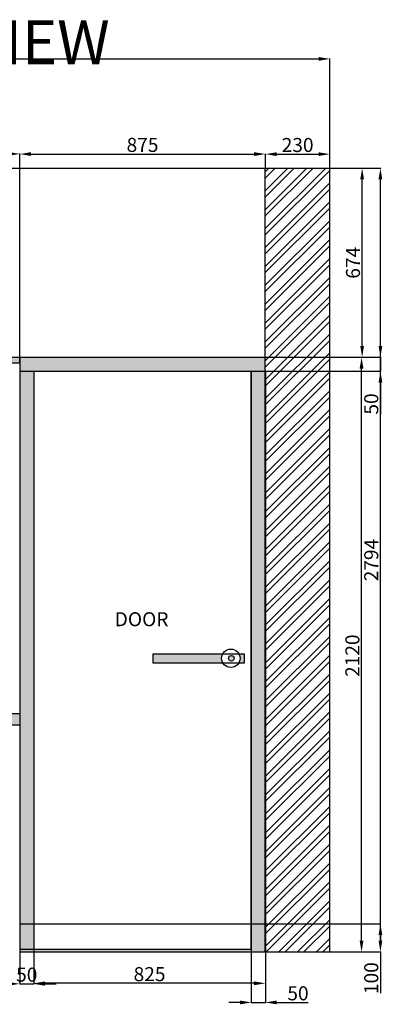
# Model space of a CAD drawing. Units: millimetres. Extents: x 144895 to 155057, y -2833 to 1092.
# Tile 2 of 4: x 147257 to 148549, y -2807 to 703. Entities that reach past the tile are written whole.
import ezdxf

# ---------------------------------------------------------------- set-up
doc = ezdxf.new("R2010")
doc.units = ezdxf.units.MM
for name, color, linetype, lineweight in [('A-ANNO-DIMS', 2, 'Continuous', 18), ('A-ANNO-TEXT', 7, 'Continuous', 18), ('A-DOOR', 4, 'Continuous', 25), ('A-ELEV', 7, 'Continuous', 25), ('A-ELEV-PATT', 252, 'Continuous', 13), ('A-WALL-PATT', 8, 'Continuous', 13)]:
    doc.layers.add(name, color=color, linetype=linetype, lineweight=lineweight)
doc.styles.get("Standard").update_dxf_attribs({"font": 'arial.ttf'})
doc.dimstyles.new('ISO-25', dxfattribs={"dimtxt": 50, "dimasz": 40, "dimexe": 1.25, "dimexo": 0.625, "dimtad": 1, "dimtxsty": 'Standard', "dimcen": 2.5, "dimadec": 0, "dimazin": 0, "dimtfac": 1, "dimtmove": 0, "dimatfit": 3, "dimfxl": 1, "dimarcsym": 0})

# ---------------------------------------------------------------- blocks, each defined once
blk = doc.blocks.new('*D13')
at = {"layer": 'A-ANNO-DIMS', "color": 0, "lineweight": -2, "transparency": 16777216}
for p, q in [((147257.5, -2621.3), (147257.5, -2735.6)), ((147307.5, -2621.3), (147307.5, -2735.6)), ((147217.5, -2734.4), (147177.5, -2734.4)), ((147257.5, -2734.4), (147307.5, -2734.4)), ((147347.5, -2734.4), (147387.5, -2734.4))]:
    blk.add_line(p, q, dxfattribs=at)
at = {"layer": 'A-ANNO-DIMS', "color": 0, "transparency": 16777216}
for points in [[(147217.5, -2727.7), (147217.5, -2741.1), (147257.5, -2734.4)], [(147347.5, -2727.7), (147347.5, -2741.1), (147307.5, -2734.4)]]:
    blk.add_solid(points, dxfattribs=at)
at = {"layer": 'Defpoints', "color": 0, "transparency": 16777216}
for p in [(147257.5, -2620.7), (147307.5, -2620.7), (147307.5, -2734.4)]:
    blk.add_point(p, dxfattribs=at)
at = {"layer": 'A-ANNO-DIMS', "color": 0, "transparency": 16777216, "insert": (147282.5, -2708.2), "char_height": 50, "attachment_point": 5}
blk.add_mtext('50', dxfattribs=at)
blk = doc.blocks.new('*D14')
at = {"layer": 'A-ANNO-DIMS', "color": 0, "lineweight": -2, "transparency": 16777216}
for p, q in [((147307.5, -2621.3), (147307.5, -2733.7)), ((148132.5, -2621.3), (148132.5, -2733.7)), ((148092.5, -2732.5), (147347.5, -2732.5))]:
    blk.add_line(p, q, dxfattribs=at)
at = {"layer": 'A-ANNO-DIMS', "color": 0, "transparency": 16777216}
for points in [[(147347.5, -2725.8), (147347.5, -2739.2), (147307.5, -2732.5)], [(148092.5, -2725.8), (148092.5, -2739.2), (148132.5, -2732.5)]]:
    blk.add_solid(points, dxfattribs=at)
at = {"layer": 'Defpoints', "color": 0, "transparency": 16777216}
for p in [(147307.5, -2620.7), (148132.5, -2620.7), (147307.5, -2732.5)]:
    blk.add_point(p, dxfattribs=at)
at = {"layer": 'A-ANNO-DIMS', "color": 0, "transparency": 16777216, "insert": (147720, -2706.3), "char_height": 50, "attachment_point": 5}
blk.add_mtext('825', dxfattribs=at)
blk = doc.blocks.new('*D22')
at = {"layer": 'A-ANNO-DIMS', "color": 0, "lineweight": -2, "ltscale": 20, "transparency": 16777216}
for p, q in [((146794.5, 173.9), (146794.5, 225.6)), ((147217.5, 224.4), (146834.5, 224.4)), ((147257.5, 173.9), (147257.5, 225.6))]:
    blk.add_line(p, q, dxfattribs=at)
at = {"layer": 'A-ANNO-DIMS', "color": 0, "ltscale": 20, "transparency": 16777216}
for points in [[(146834.5, 231), (146834.5, 217.7), (146794.5, 224.4)], [(147217.5, 231), (147217.5, 217.7), (147257.5, 224.4)]]:
    blk.add_solid(points, dxfattribs=at)
at = {"layer": 'Defpoints', "color": 0, "ltscale": 20, "transparency": 16777216}
for p in [(146794.5, 224.4), (146794.5, 173.3), (147257.5, 173.3)]:
    blk.add_point(p, dxfattribs=at)
at = {"layer": 'A-ANNO-DIMS', "color": 0, "ltscale": 20, "transparency": 16777216, "insert": (147026, 250.6), "char_height": 50, "attachment_point": 5}
blk.add_mtext('463', dxfattribs=at)
blk = doc.blocks.new('*D24')
at = {"layer": 'A-ANNO-DIMS', "color": 0, "lineweight": -2, "ltscale": 20, "transparency": 16777216}
for p, q in [((148131.9, -500.7), (148476.5, -500.7)), ((148475.2, -2580.7), (148475.2, -540.7)), ((148133.1, -2620.7), (148476.5, -2620.7))]:
    blk.add_line(p, q, dxfattribs=at)
at = {"layer": 'A-ANNO-DIMS', "color": 0, "ltscale": 20, "transparency": 16777216}
for points in [[(148468.5, -540.7), (148481.9, -540.7), (148475.2, -500.7)], [(148468.5, -2580.7), (148481.9, -2580.7), (148475.2, -2620.7)]]:
    blk.add_solid(points, dxfattribs=at)
at = {"layer": 'Defpoints', "color": 0, "ltscale": 20, "transparency": 16777216}
for p in [(148131.3, -500.7), (148475.2, -500.7), (148132.5, -2620.7)]:
    blk.add_point(p, dxfattribs=at)
at = {"layer": 'A-ANNO-DIMS', "color": 0, "ltscale": 20, "transparency": 16777216, "insert": (148449.1, -1564.5), "char_height": 50, "attachment_point": 5, "rotation": 90}
blk.add_mtext('2120', dxfattribs=at)
blk = doc.blocks.new('*D25')
at = {"layer": 'A-ANNO-DIMS', "color": 0, "lineweight": -2, "ltscale": 20, "transparency": 16777216}
for p, q in [((148131.9, 173.3), (148478.6, 173.3)), ((148477.3, -460.7), (148477.3, 133.3)), ((148131.9, -500.7), (148478.6, -500.7))]:
    blk.add_line(p, q, dxfattribs=at)
at = {"layer": 'A-ANNO-DIMS', "color": 0, "ltscale": 20, "transparency": 16777216}
for points in [[(148470.7, 133.3), (148484, 133.3), (148477.3, 173.3)], [(148470.7, -460.7), (148484, -460.7), (148477.3, -500.7)]]:
    blk.add_solid(points, dxfattribs=at)
at = {"layer": 'Defpoints', "color": 0, "ltscale": 20, "transparency": 16777216}
for p in [(148131.3, 173.3), (148477.3, 173.3), (148131.3, -500.7)]:
    blk.add_point(p, dxfattribs=at)
at = {"layer": 'A-ANNO-DIMS', "color": 0, "ltscale": 20, "transparency": 16777216, "insert": (148451.2, -163.7), "char_height": 50, "attachment_point": 5, "rotation": 90}
blk.add_mtext('674', dxfattribs=at)
blk = doc.blocks.new('*D26')
at = {"layer": 'A-ANNO-DIMS', "color": 0, "lineweight": -2, "ltscale": 20, "transparency": 16777216}
for p, q in [((147257.5, 173.9), (147257.5, 225.1)), ((147297.5, 223.8), (148092.5, 223.8)), ((148132.5, 173.9), (148132.5, 225.1))]:
    blk.add_line(p, q, dxfattribs=at)
at = {"layer": 'A-ANNO-DIMS', "color": 0, "ltscale": 20, "transparency": 16777216}
for points in [[(147297.5, 230.5), (147297.5, 217.1), (147257.5, 223.8)], [(148092.5, 230.5), (148092.5, 217.1), (148132.5, 223.8)]]:
    blk.add_solid(points, dxfattribs=at)
at = {"layer": 'Defpoints', "color": 0, "ltscale": 20, "transparency": 16777216}
for p in [(148132.5, 223.8), (147257.5, 173.3), (148132.5, 173.3)]:
    blk.add_point(p, dxfattribs=at)
at = {"layer": 'A-ANNO-DIMS', "color": 0, "ltscale": 20, "transparency": 16777216, "insert": (147695, 250), "char_height": 50, "attachment_point": 5}
blk.add_mtext('875', dxfattribs=at)
blk = doc.blocks.new('*D27')
at = {"layer": 'A-ANNO-DIMS', "color": 0, "lineweight": -2, "ltscale": 20, "transparency": 16777216}
for p, q in [((148132.5, 173.9), (148132.5, 224.8)), ((148172.5, 223.6), (148322.5, 223.6)), ((148362.5, 173.9), (148362.5, 224.8))]:
    blk.add_line(p, q, dxfattribs=at)
at = {"layer": 'A-ANNO-DIMS', "color": 0, "ltscale": 20, "transparency": 16777216}
for points in [[(148172.5, 230.2), (148172.5, 216.9), (148132.5, 223.6)], [(148322.5, 230.2), (148322.5, 216.9), (148362.5, 223.6)]]:
    blk.add_solid(points, dxfattribs=at)
at = {"layer": 'Defpoints', "color": 0, "ltscale": 20, "transparency": 16777216}
for p in [(148362.5, 223.6), (148132.5, 173.3), (148362.5, 173.3)]:
    blk.add_point(p, dxfattribs=at)
at = {"layer": 'A-ANNO-DIMS', "color": 0, "ltscale": 20, "transparency": 16777216, "insert": (148247.5, 249.7), "char_height": 50, "attachment_point": 5}
blk.add_mtext('230', dxfattribs=at)
blk = doc.blocks.new('DOOR-HANDLE')
at = {"ltscale": 20}
h = blk.add_hatch(color=256, dxfattribs=at)
h.dxf.hatch_style = 1
h.paths.add_polyline_path([(147980.9, -1557.7), (147732.7, -1557.7), (147732.7, -1591.4), (147982, -1591.4, -0.143725), (147976.8, -1573.6, -0.127114)])
h.paths.add_polyline_path([(148056.8, -1557.7), (148038.3, -1557.7, -0.127123), (148042.5, -1573.6, -0.143716), (148037.2, -1591.4), (148056.8, -1591.4)])
h.paths.add_polyline_path([(148001.6, -1573.7, 1), (148021.1, -1573.7, 1)])
blk.add_lwpolyline([(147732.7, -1557.7), (148056.8, -1557.7), (148056.8, -1591.4), (147732.7, -1591.4)], close=True, dxfattribs=at)
for centre, radius in [((148009.6, -1573.6), 32.8), ((148011.4, -1573.7), 9.79)]:
    blk.add_circle(centre, radius, dxfattribs=at)
blk = doc.blocks.new('*D46')
at = {"layer": 'A-ANNO-DIMS', "color": 0, "lineweight": -2, "ltscale": 20, "transparency": 16777216}
for p, q in [((145137.5, 173.9), (145137.5, 564.4)), ((145177.5, 563.2), (148322.5, 563.2)), ((148362.5, 173.9), (148362.5, 564.4))]:
    blk.add_line(p, q, dxfattribs=at)
at = {"layer": 'A-ANNO-DIMS', "color": 0, "ltscale": 20, "transparency": 16777216}
for points in [[(145177.5, 569.8), (145177.5, 556.5), (145137.5, 563.2)], [(148322.5, 569.8), (148322.5, 556.5), (148362.5, 563.2)]]:
    blk.add_solid(points, dxfattribs=at)
at = {"layer": 'Defpoints', "color": 0, "ltscale": 20, "transparency": 16777216}
for p in [(148362.5, 563.2), (145137.5, 173.3), (148362.5, 173.3)]:
    blk.add_point(p, dxfattribs=at)
at = {"layer": 'A-ANNO-DIMS', "color": 0, "ltscale": 20, "transparency": 16777216, "insert": (146750, 589.4), "char_height": 50, "attachment_point": 5}
blk.add_mtext('3225', dxfattribs=at)
blk = doc.blocks.new('*D47')
at = {"layer": 'A-ANNO-DIMS', "color": 0, "lineweight": -2, "ltscale": 20, "transparency": 16777216}
for p, q in [((148363.1, 173.3), (148543.7, 173.3)), ((148542.5, -2580.7), (148542.5, 133.3)), ((148363.1, -2620.7), (148543.7, -2620.7))]:
    blk.add_line(p, q, dxfattribs=at)
at = {"layer": 'A-ANNO-DIMS', "color": 0, "ltscale": 20, "transparency": 16777216}
for points in [[(148535.8, 133.3), (148549.1, 133.3), (148542.5, 173.3)], [(148535.8, -2580.7), (148549.1, -2580.7), (148542.5, -2620.7)]]:
    blk.add_solid(points, dxfattribs=at)
at = {"layer": 'Defpoints', "color": 0, "ltscale": 20, "transparency": 16777216}
for p in [(148362.5, 173.3), (148542.5, 173.3), (148362.5, -2620.7)]:
    blk.add_point(p, dxfattribs=at)
at = {"layer": 'A-ANNO-DIMS', "color": 0, "ltscale": 20, "transparency": 16777216, "insert": (148516.3, -1223.7), "char_height": 50, "attachment_point": 5, "rotation": 90}
blk.add_mtext('2794', dxfattribs=at)
blk = doc.blocks.new('*D54')
at = {"layer": 'A-ANNO-DIMS', "color": 0, "lineweight": -2, "ltscale": 20, "transparency": 16777216}
for p, q in [((147258.1, -2520.7), (148543.7, -2520.7)), ((148542.5, -2560.7), (148542.5, -2580.7)), ((147258.1, -2620.7), (148543.7, -2620.7)), ((148542.5, -2620.7), (148542.5, -2767.5))]:
    blk.add_line(p, q, dxfattribs=at)
at = {"layer": 'A-ANNO-DIMS', "color": 0, "ltscale": 20, "transparency": 16777216}
for points in [[(148535.8, -2560.7), (148549.1, -2560.7), (148542.5, -2520.7)], [(148535.8, -2580.7), (148549.1, -2580.7), (148542.5, -2620.7)]]:
    blk.add_solid(points, dxfattribs=at)
at = {"layer": 'Defpoints', "color": 0, "ltscale": 20, "transparency": 16777216}
for p in [(147257.5, -2520.7), (147257.5, -2620.7), (148542.5, -2620.7)]:
    blk.add_point(p, dxfattribs=at)
at = {"layer": 'A-ANNO-DIMS', "color": 0, "ltscale": 20, "transparency": 16777216, "insert": (148516.3, -2714.1), "char_height": 50, "attachment_point": 5, "rotation": 90}
blk.add_mtext('100', dxfattribs=at)
blk = doc.blocks.new('*D56')
at = {"layer": 'A-ANNO-DIMS', "color": 0, "lineweight": -2, "ltscale": 20, "transparency": 16777216}
for p, q in [((148542.5, -460.7), (148542.5, -420.7)), ((148131.9, -500.7), (148543.7, -500.7)), ((148542.5, -500.7), (148542.5, -550.7)), ((148083.1, -550.7), (148543.7, -550.7)), ((148542.5, -590.7), (148542.5, -703.4))]:
    blk.add_line(p, q, dxfattribs=at)
at = {"layer": 'A-ANNO-DIMS', "color": 0, "ltscale": 20, "transparency": 16777216}
for points in [[(148535.8, -460.7), (148549.1, -460.7), (148542.5, -500.7)], [(148535.8, -590.7), (148549.1, -590.7), (148542.5, -550.7)]]:
    blk.add_solid(points, dxfattribs=at)
at = {"layer": 'Defpoints', "color": 0, "ltscale": 20, "transparency": 16777216}
for p in [(148131.3, -500.7), (148082.5, -550.7), (148542.5, -550.7)]:
    blk.add_point(p, dxfattribs=at)
at = {"layer": 'A-ANNO-DIMS', "color": 0, "ltscale": 20, "transparency": 16777216, "insert": (148516.3, -667.1), "char_height": 50, "attachment_point": 5, "rotation": 90}
blk.add_mtext('50', dxfattribs=at)
blk = doc.blocks.new('*D58')
at = {"layer": 'A-ANNO-DIMS', "color": 0, "lineweight": -2, "ltscale": 20, "transparency": 16777216}
for p, q in [((148082.5, -551.3), (148082.5, -2802)), ((148132.5, -551.3), (148132.5, -2802)), ((148042.5, -2800.7), (148002.5, -2800.7)), ((148082.5, -2800.7), (148132.5, -2800.7)), ((148172.5, -2800.7), (148285.2, -2800.7))]:
    blk.add_line(p, q, dxfattribs=at)
at = {"layer": 'A-ANNO-DIMS', "color": 0, "ltscale": 20, "transparency": 16777216}
for points in [[(148042.5, -2794), (148042.5, -2807.4), (148082.5, -2800.7)], [(148172.5, -2794), (148172.5, -2807.4), (148132.5, -2800.7)]]:
    blk.add_solid(points, dxfattribs=at)
at = {"layer": 'Defpoints', "color": 0, "ltscale": 20, "transparency": 16777216}
for p in [(148082.5, -550.7), (148132.5, -550.7), (148132.5, -2800.7)]:
    blk.add_point(p, dxfattribs=at)
at = {"layer": 'A-ANNO-DIMS', "color": 0, "ltscale": 20, "transparency": 16777216, "insert": (148248.8, -2774.6), "char_height": 50, "attachment_point": 5}
blk.add_mtext('50', dxfattribs=at)

msp = doc.modelspace()

# ---------------------------------------------------------------- hatches: boundary and pattern name
at = {"layer": 'A-ELEV-PATT', "ltscale": 20}
h = msp.add_hatch(color=256, dxfattribs=at)
h.dxf.hatch_style = 1
h.paths.add_polyline_path([(146350.96, -520.704), (146310.96, -520.704), (146310.96, -1550.704), (146350.96, -1550.704)])
h.paths.add_polyline_path([(145867.46, 173.296), (145817.46, 173.296), (145817.46, -500.704), (145867.46, -500.704)])
h.paths.add_polyline_path([(145867.46, -500.704), (145367.46, -500.704), (145367.46, -520.704), (145867.46, -520.704)])
h.paths.add_polyline_path([(147257.46, -500.704), (146794.46, -500.704), (146794.46, -520.704), (147257.46, -520.704)])
h.paths.add_polyline_path([(147257.46, -1770.704), (146656.275, -1770.704), (146656.07, -1810.704), (146847.46, -1810.704), (147257.46, -1810.704)])
h.paths.add_polyline_path([(148132.46, -550.704), (148082.46, -550.704), (148082.46, -2610.704), (147307.46, -2610.704), (147307.46, -2620.704), (148132.46, -2620.704)])
h.paths.add_polyline_path([(146109.393, -1080.003), (146541.794, -1080.003), (146541.794, -976.968), (146109.393, -976.968)], flags=9)
h = msp.add_hatch(color=256, dxfattribs=at)
h.dxf.hatch_style = 1
h.paths.add_polyline_path([(147307.46, -550.704), (147257.46, -550.704), (147257.46, -2620.704), (147307.46, -2620.704)])
h.paths.add_polyline_path([(148132.46, -500.704), (147257.46, -500.704), (147257.46, -550.704), (148132.46, -550.704)])
h.paths.add_polyline_path([(148132.46, -550.704), (148082.46, -550.704), (148082.46, -2620.704), (148132.46, -2620.704)])
at = {"layer": 'A-WALL-PATT'}
h = msp.add_hatch(dxfattribs=at)
h.set_pattern_fill('ANSI32', color=256, scale=5)
h.paths.add_polyline_path([(148132.46, -2620.704), (148362.46, -2620.704), (148362.46, 173.296), (148132.46, 173.296)])

# ---------------------------------------------------------------- linework, layer by layer
at = {"layer": 'A-ELEV'}
for p, q in [((145137.46, 173.296), (148362.46, 173.296)), ((147257.46, -520.704), (147257.46, 173.296)), ((148132.46, -2620.704), (148132.46, 173.296)), ((148362.46, -2620.704), (148362.46, 173.296)), ((145367.46, -500.704), (148131.298, -500.704)), ((146794.46, -520.704), (147257.46, -520.704)), ((147257.46, -500.704), (147257.46, -2620.704)), ((147257.46, -550.704), (148132.46, -550.704)), ((147307.46, -550.704), (147307.46, -2620.704)), ((148082.46, -2610.704), (148082.46, -550.704)), ((145367.46, -1770.704), (147257.46, -1770.704)), ((146847.46, -1810.704), (147257.46, -1810.704)), ((147257.46, -2610.704), (148082.46, -2610.704)), ((147257.46, -2620.704), (148362.46, -2620.704))]:
    msp.add_line(p, q, dxfattribs=at)

# ---------------------------------------------------------------- block references
at = {"layer": 'A-DOOR'}
msp.add_blockref('DOOR-HANDLE', (0, 0), dxfattribs=at)

# ---------------------------------------------------------------- texts
at = {"layer": 'A-ANNO-TEXT', "attachment_point": 1}
for s, width, gutter_width, insert, char_height in [('OVER VIEW', 9064.84564, 39.102, (146489.911, 700.132), 156.408), ('DOOR', 2897.81963, 12.5, (147595.941, -1409.526), 50)]:
    msp.add_mtext_dynamic_manual_height_columns(s, width=width, gutter_width=gutter_width, heights=[0], dxfattribs=dict(at, insert=insert, char_height=char_height))

# ---------------------------------------------------------------- dimensions: what is measured, and where the dimension line sits
at = {"layer": 'A-ANNO-DIMS', "ltscale": 20}
for base, p1, p2, override, picture, middle in [((148362.46, 563.182), (145137.46, 173.296), (148362.46, 173.296), {"dimdec": 0, "dimlfac": 1, "dimrnd": 0, "dimzin": 0, "dimdsep": 46, "dimlunit": 2}, '*D46', (146749.96, 589.353)), ((146794.46, 224.38), (147257.46, 173.296), (146794.46, 173.296), {"dimclrd": 0, "dimclre": 0, "dimclrt": 0}, '*D22', (147025.96, 250.551)), ((148132.46, 223.813), (147257.46, 173.296), (148132.46, 173.296), {"dimclrd": 0, "dimclre": 0, "dimclrt": 0}, '*D26', (147694.96, 249.967)), ((148362.46, 223.551), (148132.46, 173.296), (148362.46, 173.296), {"dimclrd": 0, "dimclre": 0, "dimclrt": 0}, '*D27', (148247.46, 249.721)), ((148132.46, -2800.704), (148082.46, -550.704), (148132.46, -550.704), {"dimdec": 0, "dimlfac": 1, "dimrnd": 0, "dimzin": 0, "dimdsep": 46, "dimlunit": 2}, '*D58', (148248.812, -2774.55))]:
    dim = msp.add_linear_dim(base=base, p1=p1, p2=p2, dimstyle='ISO-25', override=override, dxfattribs=at)
    dim.commit()
    dim.dimension.update_dxf_attribs({"geometry": picture, "text_midpoint": middle})
for base, p1, p2, override, picture, middle in [((148477.343, 173.296), (148131.298, -500.704), (148131.298, 173.296), {"dimclrd": 0, "dimclre": 0, "dimclrt": 0}, '*D25', (148451.19, -163.704)), ((148542.46, 173.296), (148362.46, -2620.704), (148362.46, 173.296), {"dimdec": 0, "dimlfac": 1, "dimrnd": 0, "dimzin": 0, "dimdsep": 46, "dimlunit": 2}, '*D47', (148516.307, -1223.704)), ((148542.46, -550.704), (148131.298, -500.704), (148082.46, -550.704), {"dimdec": 0, "dimlfac": 1, "dimrnd": 0, "dimzin": 0, "dimdsep": 46, "dimlunit": 2}, '*D56', (148516.307, -667.055)), ((148542.46, -2620.704), (147257.46, -2520.704), (147257.46, -2620.704), {"dimdec": 0, "dimlfac": 1, "dimrnd": 0, "dimzin": 0, "dimdsep": 46, "dimlunit": 2}, '*D54', (148516.307, -2714.126))]:
    dim = msp.add_linear_dim(base=base, p1=p1, p2=p2, angle=90, dimstyle='ISO-25', override=override, dxfattribs=at)
    dim.commit()
    dim.dimension.update_dxf_attribs({"geometry": picture, "text_midpoint": middle})
dim = msp.add_linear_dim(base=(148475.214, -500.704), p1=(148132.46, -2620.704), p2=(148131.298, -500.704), angle=90, dimstyle='ISO-25', override={"dimclrd": 0, "dimclre": 0, "dimclrt": 0}, dxfattribs=at)
dim.commit()
dim.dimension.update_dxf_attribs({"geometry": '*D24', "text_midpoint": (148475.214, -1564.504), "dimtype": 160})
at = {"layer": 'A-ANNO-DIMS'}
dim = msp.add_linear_dim(base=(147307.46, -2734.384), p1=(147257.46, -2620.704), p2=(147307.46, -2620.704), dimstyle='ISO-25', override={"dimclrd": 0, "dimclre": 0, "dimclrt": 0}, dxfattribs=at)
dim.commit()
dim.dimension.update_dxf_attribs({"geometry": '*D13', "text_midpoint": (147282.46, -2734.384), "dimtype": 160})
dim = msp.add_linear_dim(base=(147307.46, -2732.484), p1=(148132.46, -2620.704), p2=(147307.46, -2620.704), dimstyle='ISO-25', override={"dimclrd": 0, "dimclre": 0, "dimclrt": 0}, dxfattribs=at)
dim.commit()
dim.dimension.update_dxf_attribs({"geometry": '*D14', "text_midpoint": (147719.96, -2706.331)})

doc.saveas('drawing.dxf')
